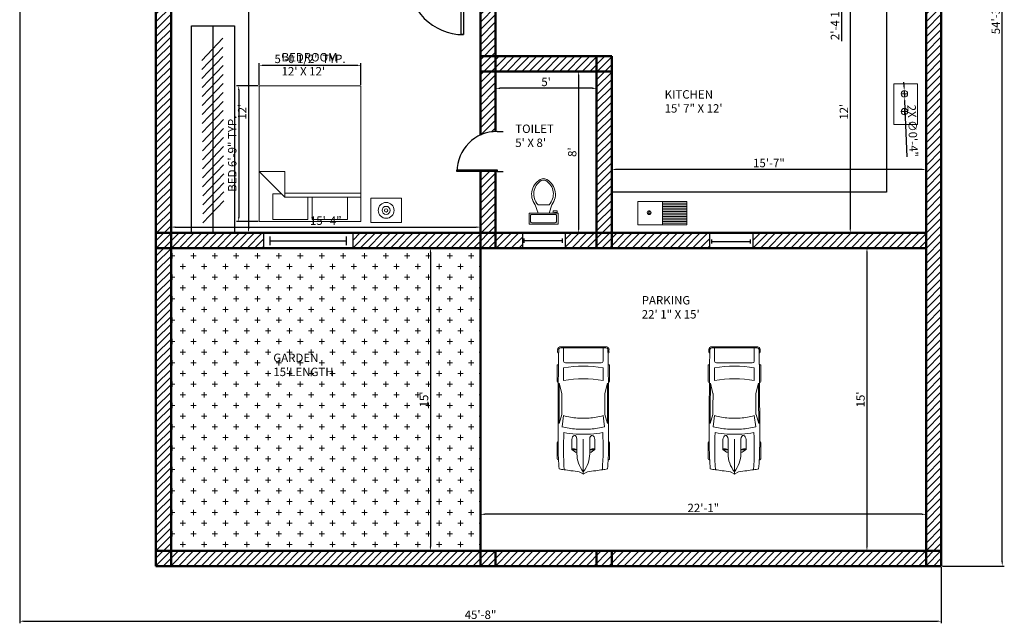
# Model space of a CAD drawing. Units: millimetres. Extents: x 2829 to 4029, y 962 to 1687.
# Tile 5 of 7: x 3444 to 4029, y 962 to 1321. Entities that reach past the tile are written whole.
import ezdxf

# ---------------------------------------------------------------- set-up
doc = ezdxf.new("R2010")
doc.units = ezdxf.units.MM
for name, color, linetype, lineweight in [('A-ANNO-DIMS', 140, 'Continuous', 18), ('A-AREA-IDEN', 190, 'Continuous', 25), ('A-EQPM', 90, 'Continuous', 18), ('A-FLOR-CASE', 90, 'Continuous', 25), ('A-FLOR-CASE-PATT', 90, 'Continuous', 13), ('A-FLOR-FIXT', 90, 'Continuous', 18), ('A-FLOR-FIXT-PATT', 90, 'Continuous', 13), ('A-WALL-PATT', 2, 'Continuous', 13), ('C-PRKG-VEHS', 90, 'Continuous', 18), ('doors', 10, 'Continuous', 25), ('furniture', 90, 'Continuous', 18), ('walls', 50, 'Continuous', 50), ('windows', 30, 'Continuous', 25)]:
    doc.layers.add(name, color=color, linetype=linetype, lineweight=lineweight)
doc.layers.add('L-PLNT-PATT', color=143, linetype='Continuous', lineweight=13, true_color=0x7aafdf)
doc.styles.get("Standard").update_dxf_attribs({"font": 'arial.ttf'})
doc.dimstyles.new('ISO-25', dxfattribs={"dimtxt": 5, "dimasz": 2.5, "dimexe": 1.25, "dimexo": 0.625, "dimtad": 1, "dimdec": 0, "dimlunit": 3, "dimtxsty": 'Standard', "dimcen": 2.5, "dimadec": 0, "dimazin": 0, "dimtfac": 1, "dimtdec": 0, "dimtmove": 0, "dimatfit": 3, "dimfxl": 1, "dimarcsym": 0})

# ---------------------------------------------------------------- blocks, each defined once
blk = doc.blocks.new('*U2')
for p, q in [((0, 0), (0, -6)), ((40, 0), (40, -6))]:
    blk.add_line(p, q)
blk.add_lwpolyline([(0, 0), (0, 40), (1.75, 40), (1.75, 0)], close=True)
blk.add_arc((0, 0), 40, 0, 90)
blk = doc.blocks.new('*U32')
for p, q in [((0, 4), (0, 0)), ((0, 2), (36, 2)), ((36, 4), (36, 0))]:
    blk.add_line(p, q)
blk = doc.blocks.new('*U33')
for p, q in [((0, 4), (0, 0)), ((0, 2), (36, 2)), ((36, 4), (36, 0))]:
    blk.add_line(p, q)
blk = doc.blocks.new('Bed - Queen')
for p, q in [((0, -80.00003), (0, 0)), ((0, 0), (59.99999, 0)), ((59.99999, 0), (59.99999, -80.00003)), ((7.99999, -1.2), (28.79998, -1.2)), ((7.99999, -14.4), (7.99999, -1.2)), ((28.79998, -1.2), (28.79998, -14.4)), ((31.19999, -1.2), (51.99999, -1.2)), ((31.19999, -14.4), (31.19999, -1.2)), ((51.99999, -1.2), (51.99999, -16.4)), ((0, -14.4), (44.8, -14.4)), ((44.8, -16.8), (0, -16.8)), ((59.99999, -29.6), (44.8, -14.4)), ((44.8, -14.4), (44.8, -29.6)), ((51.99999, -16.4), (46.79936, -16.4)), ((44.8, -29.6), (59.99999, -29.6)), ((59.99999, -80.00003), (0, -80.00003))]:
    blk.add_line(p, q)
blk = doc.blocks.new('*U35')
for p, q in [((21.1, 37.4), (21.1, 36.8)), ((46.6, 38.9), (22.4, 38.9)), ((47.8, 37.4), (47.8, 37.4)), ((70, 31.5), (86.4, 29.4)), ((88, 31.9), (74.8, 35.9)), ((134.3, 35.6), (119.3, 31.8)), ((135.5, 37.1), (135.5, 37.4)), ((136.7, 38.9), (160.9, 38.9)), ((138.4, 29.4), (157.2, 29.4)), ((162.1, 37.4), (162.1, 36.8)), ((186.5, 29.4), (167, 29.4)), ((186.5, -33.5), (186.5, 33.5)), ((188.4, -32.8), (188.4, 32.8)), ((32.3, 11.6), (36.1, 17.2)), ((36.1, 17.2), (50.9, 17.2)), ((164.5, 26.4), (164.5, -26.4)), ((3.3, 6.1), (0.1, 0.4)), ((29.8, 9.5), (51.7, 9.5)), ((32.1, 9.5), (32.1, 11.2)), ((58.9, -10.8), (58.9, 10.8)), ((66.6, -10.5), (66.6, 10.5)), ((82.7, 8.5), (82.7, -8.5)), ((186.5, -10.5), (186.5, 10.5)), ((0, 0), (51.7, 0)), ((0.1, -0.4), (3.3, -6.1)), ((29.8, -9.5), (51.7, -9.5)), ((32.1, -9.5), (32.1, -11.2)), ((32.3, -11.6), (36.1, -17.2)), ((36.1, -17.2), (50.9, -17.2)), ((21.1, -37.4), (21.1, -36.8)), ((46.6, -38.9), (22.4, -38.9)), ((47.8, -37.4), (47.8, -37.4)), ((86.4, -29.4), (70, -31.5)), ((88, -31.9), (74.8, -35.9)), ((134.3, -35.6), (119.3, -31.8)), ((135.5, -37.1), (135.5, -37.4)), ((136.7, -38.9), (160.9, -38.9)), ((157.2, -29.4), (138.4, -29.4)), ((162.1, -37.4), (162.1, -36.8)), ((167, -29.4), (186.5, -29.4))]:
    blk.add_line(p, q)
for centre, major_axis, ratio, start_param, end_param in [((266, -27.5), (0, 313.3), 0.842304, 1.367076, 1.39176), ((37.5, -594), (0, -623.3), 0.842304, 3.096046, 3.200911), ((41.2, -490.9), (0, 528.2), 0.842304, 0.00281, 0.075598), ((22.4, 37.4), (0, -1.48), 0.842304, 3.141593, 4.712389), ((64.5, -10555.6), (0, 10593), 0.842304, -0.013397, 0.002797), ((46.6, 37.4), (0, 1.48), 0.842304, -1.570796, 0), ((135.3, 5.4), (0, 81.8), 0.842304, 1.245306, 1.50788), ((64.5, -10555.6), (0, -10591.5), 0.842304, 3.133765, 3.140441), ((149.6, 2.8), (0, -79.6), 0.842304, 4.372215, 4.640744), ((95.8, -3666.4), (0, -3698.2), 0.842304, 3.134049, 3.144098), ((136.7, 37.4), (0, -1.48), 0.842304, 3.141593, 4.712389), ((17.1, 0), (0, 147), 0.842304, 4.511394, 4.913384), ((35.9, 0), (0, 147), 0.842304, 4.511394, 4.913384), ((160.9, 37.4), (0, 1.48), 0.842304, -1.570796, 0), ((167, 26.4), (0, 2.96), 0.842304, 0, 1.570796), ((180.6, 35.8), (0, 2.22), 0.842304, -0.013017, 1.249894), ((64.5, -10556.4), (0, 10595.3), 0.842304, -0.013397, -0.013017), ((184, 32.8), (0, -5.25), 0.842304, 1.570796, 3.128196), ((184, 33.5), (0, -2.96), 0.842304, 1.570796, 3.128196), ((-204.5, 52.4), (0, -251), 0.842304, 1.385369, 1.434372), ((259.2, -27.5), (0, -305.3), 0.842304, 4.528606, 4.561838), ((13, 17), (0, 27.4), 0.842304, 4.435146, 4.718221), ((14.2, 17), (0, 27.4), 0.842304, 4.435146, 4.718221), ((50.8, 13.3), (6.34, -0.36), 0.603834, -1.395552, 1.581315), ((134.4, 5.4), (0, -89.8), 0.842304, 4.449482, 4.652344), ((0.6, 0), (0, -0.74), 0.842304, 4.131459, 5.293319), ((29.8, -46.7), (0, 56.2), 0.842304, 0, 0.590319), ((32.7, 11.2), (0, 0.74), 0.842304, 0.879714, 1.570796), ((-204.5, -52.4), (0, 251), 0.842304, -1.434372, -1.385369), ((29.8, 46.7), (0, 56.2), 0.842304, 2.551274, 3.141593), ((32.7, -11.2), (0, -0.74), 0.842304, 4.712389, 5.403472), ((13, -17), (0, -27.4), 0.842304, 1.564964, 1.848039), ((14.2, -17), (0, -27.4), 0.842304, 1.564964, 1.848039), ((134.4, -5.4), (0, -89.8), 0.842304, -1.510751, -1.307889), ((135.3, -5.4), (0, -81.8), 0.842304, -1.50788, -1.245306), ((149.6, -2.8), (0, -79.6), 0.842304, -1.499151, -1.230623), ((259.2, 27.5), (0, 305.3), 0.842304, 1.721348, 1.754579), ((266, 27.5), (0, 313.3), 0.842304, 1.749832, 1.774517), ((37.5, 594), (0, -623.3), 0.842304, -0.059319, 0.045547), ((167, -26.4), (0, -2.96), 0.842304, 4.712389, 6.283185), ((41.2, 490.9), (0, -528.2), 0.842304, -0.075598, -0.00281), ((22.4, -37.4), (0, 1.48), 0.842304, 1.570796, 3.141593), ((64.5, 10555.6), (0, 10593), 0.842304, 3.138796, 3.15499), ((46.6, -37.4), (0, -1.48), 0.842304, 0, 1.570796), ((64.5, 10555.6), (0, -10591.5), 0.842304, 0.001152, 0.007828), ((95.8, 3666.4), (0, -3698.2), 0.842304, -0.002505, 0.007544), ((136.7, -37.4), (0, -1.48), 0.842304, -1.570796, 0), ((160.9, -37.4), (0, 1.48), 0.842304, 3.141593, 4.712389), ((180.6, -35.8), (0, -2.22), 0.842304, -1.249894, 0.013017), ((64.5, 10556.4), (0, 10595.3), 0.842304, 3.15461, 3.15499), ((184, -32.8), (0, -5.25), 0.842304, 0.013397, 1.570796), ((184, -33.5), (0, 2.96), 0.842304, 3.15499, 4.712389)]:
    blk.add_ellipse(centre, major_axis=major_axis, ratio=ratio, start_param=start_param, end_param=end_param)
at = {"extrusion": (0, 0, -1)}
blk.add_ellipse((50.8, -13.3), major_axis=(6.34, 0.36), ratio=0.603834, start_param=-1.395552, end_param=1.581315, dxfattribs=at)
blk = doc.blocks.new('Toilet - top')
for p, q in [((9.5, -6), (9.5, -2)), ((-10, -8.5), (-8, -8.5)), ((-10, -9.5), (-10, -8.5)), ((-7, -9.5), (-10, -9.5)), ((-8, -8.5), (-8, -8)), ((-7, -8), (-7, -9.5)), ((-4, -8), (-6, -14)), ((4, -14), (-4, -14)), ((4, -8), (6, -14))]:
    blk.add_line(p, q)
blk.add_lwpolyline([(10.5, -8), (10.5, 0), (-10.5, 0), (-10.5, -8)], close=True)
for points in [[(-9.5, -2), (-9.5, -6)], [(8.5, -1), (-8.5, -1)], [(-8.5, -7), (8.5, -7)]]:
    blk.add_lwpolyline(points)
for centre, radius, start, end in [((-8.62, -1.88), 0.884, 81.8699, 188.1301), ((-8.62, -6.12), 0.884, 171.8699, 278.1301), ((8.62, -1.88), 0.884, 351.8699, 98.1301), ((8.62, -6.12), 0.884, 261.8699, 8.1301), ((3.52, -21.58), 12.17, 141.46911, 247.97143), ((4.2, -21.82), 11.33, 136.36773, 238.94682), ((-3.52, -21.58), 12.17, 292.02843, 38.53071), ((-4.2, -21.82), 11.33, 301.05301, 43.63209), ((0, -27.88), 4, 245.73182, 294.26817), ((0, -29), 4, 254.86053, 285.13947)]:
    blk.add_arc(centre, radius, start, end)
blk = doc.blocks.new('*D42')
at = {"layer": 'A-ANNO-DIMS', "color": 0, "lineweight": -2, "transparency": 16777216}
for p, q in [((3776.63, 1290.27), (3777.26, 1290.27)), ((3776.01, 1287.77), (3776.01, 1196.77)), ((3776.63, 1194.27), (3777.26, 1194.27))]:
    blk.add_line(p, q, dxfattribs=at)
at = {"layer": 'A-ANNO-DIMS', "color": 0, "transparency": 16777216}
for points in [[(3775.59, 1287.77), (3776.42, 1287.77), (3776.01, 1290.27)], [(3775.59, 1196.77), (3776.42, 1196.77), (3776.01, 1194.27)]]:
    blk.add_solid(points, dxfattribs=at)
at = {"layer": 'Defpoints', "color": 0, "transparency": 16777216}
for p in [(3776.01, 1290.27), (3776.01, 1194.27), (3776.01, 1194.27)]:
    blk.add_point(p, dxfattribs=at)
at = {"layer": 'A-ANNO-DIMS', "color": 0, "transparency": 16777216, "insert": (3772.83, 1242.27), "char_height": 5, "attachment_point": 5, "rotation": 90}
blk.add_mtext("8'", dxfattribs=at)
blk = doc.blocks.new('*D43')
at = {"layer": 'A-ANNO-DIMS', "color": 0, "lineweight": -2, "transparency": 16777216}
for p, q in [((3726.66, 1282.83), (3726.66, 1278.94)), ((3786.66, 1282.83), (3786.66, 1278.94)), ((3784.16, 1280.19), (3729.16, 1280.19))]:
    blk.add_line(p, q, dxfattribs=at)
at = {"layer": 'A-ANNO-DIMS', "color": 0, "transparency": 16777216}
for points in [[(3729.16, 1280.61), (3729.16, 1279.78), (3726.66, 1280.19)], [(3784.16, 1280.61), (3784.16, 1279.78), (3786.66, 1280.19)]]:
    blk.add_solid(points, dxfattribs=at)
at = {"layer": 'Defpoints', "color": 0, "transparency": 16777216}
for p in [(3726.66, 1283.46), (3786.66, 1283.46), (3726.66, 1280.19)]:
    blk.add_point(p, dxfattribs=at)
at = {"layer": 'A-ANNO-DIMS', "color": 0, "transparency": 16777216, "insert": (3756.66, 1283.36), "char_height": 5, "attachment_point": 5}
blk.add_mtext("5'", dxfattribs=at)
blk = doc.blocks.new('*D44')
at = {"layer": 'A-ANNO-DIMS', "color": 0, "lineweight": -2, "transparency": 16777216}
for p, q in [((3947.43, 1182.77), (3947.43, 1007.77)), ((3947.78, 1185.27), (3948.68, 1185.27)), ((3947.78, 1005.27), (3948.68, 1005.27))]:
    blk.add_line(p, q, dxfattribs=at)
at = {"layer": 'A-ANNO-DIMS', "color": 0, "transparency": 16777216}
for points in [[(3947.01, 1182.77), (3947.84, 1182.77), (3947.43, 1185.27)], [(3947.01, 1007.77), (3947.84, 1007.77), (3947.43, 1005.27)]]:
    blk.add_solid(points, dxfattribs=at)
at = {"layer": 'Defpoints', "color": 0, "transparency": 16777216}
for p in [(3947.15, 1185.27), (3947.15, 1005.27), (3947.43, 1005.27)]:
    blk.add_point(p, dxfattribs=at)
at = {"layer": 'A-ANNO-DIMS', "color": 0, "transparency": 16777216, "insert": (3944.25, 1095.27), "char_height": 5, "attachment_point": 5, "rotation": 90}
blk.add_mtext("15'", dxfattribs=at)
blk = doc.blocks.new('*D45')
at = {"layer": 'A-ANNO-DIMS', "color": 0, "lineweight": -2, "transparency": 16777216}
for p, q in [((3717.66, 1027.63), (3717.66, 1028.25)), ((3980.16, 1027), (3720.16, 1027)), ((3982.66, 1027.63), (3982.66, 1028.25))]:
    blk.add_line(p, q, dxfattribs=at)
at = {"layer": 'A-ANNO-DIMS', "color": 0, "transparency": 16777216}
for points in [[(3720.16, 1027.42), (3720.16, 1026.59), (3717.66, 1027)], [(3980.16, 1027.42), (3980.16, 1026.59), (3982.66, 1027)]]:
    blk.add_solid(points, dxfattribs=at)
at = {"layer": 'Defpoints', "color": 0, "transparency": 16777216}
for p in [(3717.66, 1027), (3717.66, 1027), (3982.66, 1027)]:
    blk.add_point(p, dxfattribs=at)
at = {"layer": 'A-ANNO-DIMS', "color": 0, "transparency": 16777216, "insert": (3850.16, 1030.14), "char_height": 5, "attachment_point": 5}
blk.add_mtext('22\'-1"', dxfattribs=at)
blk = doc.blocks.new('*D46')
at = {"layer": 'A-ANNO-DIMS', "color": 0, "lineweight": -2, "transparency": 16777216}
for p, q in [((3685.57, 1185.27), (3689.13, 1185.27)), ((3687.88, 1182.77), (3687.88, 1007.77)), ((3685.57, 1005.27), (3689.13, 1005.27))]:
    blk.add_line(p, q, dxfattribs=at)
at = {"layer": 'A-ANNO-DIMS', "color": 0, "transparency": 16777216}
for points in [[(3687.47, 1182.77), (3688.3, 1182.77), (3687.88, 1185.27)], [(3687.47, 1007.77), (3688.3, 1007.77), (3687.88, 1005.27)]]:
    blk.add_solid(points, dxfattribs=at)
at = {"layer": 'Defpoints', "color": 0, "transparency": 16777216}
for p in [(3684.95, 1185.27), (3684.95, 1005.27), (3687.88, 1005.27)]:
    blk.add_point(p, dxfattribs=at)
at = {"layer": 'A-ANNO-DIMS', "color": 0, "transparency": 16777216, "insert": (3684.71, 1095.27), "char_height": 5, "attachment_point": 5, "rotation": 90}
blk.add_mtext("15'", dxfattribs=at)
blk = doc.blocks.new('*D47')
at = {"layer": 'A-ANNO-DIMS', "color": 0, "lineweight": -2, "transparency": 16777216}
for p, q in [((3579.16, 1338.27), (3580.98, 1338.27)), ((3579.73, 1335.77), (3579.73, 1196.77)), ((3579.16, 1194.27), (3580.98, 1194.27))]:
    blk.add_line(p, q, dxfattribs=at)
at = {"layer": 'A-ANNO-DIMS', "color": 0, "transparency": 16777216}
for points in [[(3579.31, 1335.77), (3580.15, 1335.77), (3579.73, 1338.27)], [(3579.31, 1196.77), (3580.15, 1196.77), (3579.73, 1194.27)]]:
    blk.add_solid(points, dxfattribs=at)
at = {"layer": 'Defpoints', "color": 0, "transparency": 16777216}
for p in [(3578.53, 1338.27), (3578.53, 1194.27), (3579.73, 1194.27)]:
    blk.add_point(p, dxfattribs=at)
at = {"layer": 'A-ANNO-DIMS', "color": 0, "transparency": 16777216, "insert": (3576.59, 1266.27), "char_height": 5, "attachment_point": 5, "rotation": 90}
blk.add_mtext("12'", dxfattribs=at)
blk = doc.blocks.new('*D48')
at = {"layer": 'A-ANNO-DIMS', "color": 0, "lineweight": -2, "transparency": 16777216}
for p, q in [((3533.66, 1199.99), (3533.66, 1196.45)), ((3536.16, 1197.7), (3715.16, 1197.7)), ((3717.66, 1198.33), (3717.66, 1198.95))]:
    blk.add_line(p, q, dxfattribs=at)
at = {"layer": 'A-ANNO-DIMS', "color": 0, "transparency": 16777216}
for points in [[(3536.16, 1198.12), (3536.16, 1197.28), (3533.66, 1197.7)], [(3715.16, 1198.12), (3715.16, 1197.28), (3717.66, 1197.7)]]:
    blk.add_solid(points, dxfattribs=at)
at = {"layer": 'Defpoints', "color": 0, "transparency": 16777216}
for p in [(3533.66, 1200.61), (3717.66, 1197.7), (3717.66, 1197.7)]:
    blk.add_point(p, dxfattribs=at)
at = {"layer": 'A-ANNO-DIMS', "color": 0, "transparency": 16777216, "insert": (3625.66, 1200.88), "char_height": 5, "attachment_point": 5}
blk.add_mtext('15\'-4"', dxfattribs=at)
blk = doc.blocks.new('*D55')
at = {"layer": 'A-ANNO-DIMS', "color": 0, "lineweight": -2, "transparency": 16777216}
for p, q in [((3937.54, 1338.27), (3936.26, 1338.27)), ((3937.51, 1335.77), (3937.51, 1196.77)), ((3937.54, 1194.27), (3936.26, 1194.27))]:
    blk.add_line(p, q, dxfattribs=at)
at = {"layer": 'A-ANNO-DIMS', "color": 0, "transparency": 16777216}
for points in [[(3937.1, 1335.77), (3937.93, 1335.77), (3937.51, 1338.27)], [(3937.1, 1196.77), (3937.93, 1196.77), (3937.51, 1194.27)]]:
    blk.add_solid(points, dxfattribs=at)
at = {"layer": 'Defpoints', "color": 0, "transparency": 16777216}
for p in [(3938.16, 1338.27), (3937.51, 1194.27), (3938.16, 1194.27)]:
    blk.add_point(p, dxfattribs=at)
at = {"layer": 'A-ANNO-DIMS', "color": 0, "transparency": 16777216, "insert": (3934.38, 1266.27), "char_height": 5, "attachment_point": 5, "rotation": 90}
blk.add_mtext("12'", dxfattribs=at)
blk = doc.blocks.new('*D56')
at = {"layer": 'A-ANNO-DIMS', "color": 0, "lineweight": -2, "transparency": 16777216}
for p, q in [((3795.66, 1231.66), (3795.66, 1230.72)), ((3980.16, 1231.97), (3798.16, 1231.97)), ((3982.66, 1231.66), (3982.66, 1230.72))]:
    blk.add_line(p, q, dxfattribs=at)
at = {"layer": 'A-ANNO-DIMS', "color": 0, "transparency": 16777216}
for points in [[(3798.16, 1232.39), (3798.16, 1231.55), (3795.66, 1231.97)], [(3980.16, 1232.39), (3980.16, 1231.55), (3982.66, 1231.97)]]:
    blk.add_solid(points, dxfattribs=at)
at = {"layer": 'Defpoints', "color": 0, "transparency": 16777216}
for p in [(3795.66, 1232.29), (3795.66, 1231.97), (3982.66, 1232.29)]:
    blk.add_point(p, dxfattribs=at)
at = {"layer": 'A-ANNO-DIMS', "color": 0, "transparency": 16777216, "insert": (3889.16, 1235.15), "char_height": 5, "attachment_point": 5}
blk.add_mtext('15\'-7"', dxfattribs=at)
blk = doc.blocks.new('COOKTOP-BURNER-LARGE')
for p, q in [((0, 1.91), (3.83, 1.91)), ((1.91, 3.83), (1.91, 0))]:
    blk.add_line(p, q)
blk.add_circle((1.91, 1.91), 1.91)
blk = doc.blocks.new('*D68')
at = {"layer": 'A-ANNO-DIMS', "color": 0, "lineweight": -2, "transparency": 16777216}
for p, q in [((3923.13, 1382.67), (3933.53, 1382.67)), ((3932.28, 1380.17), (3932.28, 1356.73)), ((3923.13, 1354.23), (3933.53, 1354.23)), ((3932.28, 1354.23), (3932.28, 1308.27))]:
    blk.add_line(p, q, dxfattribs=at)
at = {"layer": 'A-ANNO-DIMS', "color": 0, "transparency": 16777216}
for points in [[(3931.86, 1380.17), (3932.7, 1380.17), (3932.28, 1382.67)], [(3931.86, 1356.73), (3932.7, 1356.73), (3932.28, 1354.23)]]:
    blk.add_solid(points, dxfattribs=at)
at = {"layer": 'Defpoints', "color": 0, "transparency": 16777216}
for p in [(3922.51, 1382.67), (3922.51, 1354.23), (3932.28, 1354.23)]:
    blk.add_point(p, dxfattribs=at)
at = {"layer": 'A-ANNO-DIMS', "color": 0, "transparency": 16777216, "insert": (3929.07, 1330), "char_height": 5, "attachment_point": 5, "rotation": 90}
blk.add_mtext('2\'-4 1/2" TYP.', dxfattribs=at)
blk = doc.blocks.new('*D71')
at = {"layer": 'A-ANNO-DIMS', "color": 0, "lineweight": -2, "transparency": 16777216}
for p, q in [((3585.37, 1281.74), (3572.63, 1281.74)), ((3573.88, 1279.24), (3573.88, 1203.47)), ((3585.37, 1200.97), (3572.63, 1200.97))]:
    blk.add_line(p, q, dxfattribs=at)
at = {"layer": 'A-ANNO-DIMS', "color": 0, "transparency": 16777216}
for points in [[(3573.47, 1279.24), (3574.3, 1279.24), (3573.88, 1281.74)], [(3573.47, 1203.47), (3574.3, 1203.47), (3573.88, 1200.97)]]:
    blk.add_solid(points, dxfattribs=at)
at = {"layer": 'Defpoints', "color": 0, "transparency": 16777216}
for p in [(3586, 1281.74), (3573.88, 1200.97), (3586, 1200.97)]:
    blk.add_point(p, dxfattribs=at)
at = {"layer": 'A-ANNO-DIMS', "color": 0, "transparency": 16777216, "insert": (3570.7, 1241.35), "char_height": 5, "attachment_point": 5, "rotation": 90}
blk.add_mtext('BED 6\'-9" TYP.', dxfattribs=at)
blk = doc.blocks.new('*D72')
at = {"layer": 'A-ANNO-DIMS', "color": 0, "lineweight": -2, "transparency": 16777216}
for p, q in [((3586, 1282.36), (3586, 1295.1)), ((3644.08, 1293.85), (3588.5, 1293.85)), ((3646.58, 1282.36), (3646.58, 1295.1))]:
    blk.add_line(p, q, dxfattribs=at)
at = {"layer": 'A-ANNO-DIMS', "color": 0, "transparency": 16777216}
for points in [[(3588.5, 1294.27), (3588.5, 1293.44), (3586, 1293.85)], [(3644.08, 1294.27), (3644.08, 1293.44), (3646.58, 1293.85)]]:
    blk.add_solid(points, dxfattribs=at)
at = {"layer": 'Defpoints', "color": 0, "transparency": 16777216}
for p in [(3586, 1293.85), (3586, 1281.74), (3646.58, 1281.74)]:
    blk.add_point(p, dxfattribs=at)
at = {"layer": 'A-ANNO-DIMS', "color": 0, "transparency": 16777216, "insert": (3616.29, 1297.06), "char_height": 5, "attachment_point": 5}
blk.add_mtext('5\'-0 1/2" TYP.', dxfattribs=at)
blk = doc.blocks.new('*D92')
at = {"layer": 'A-ANNO-DIMS', "color": 0, "lineweight": -2, "transparency": 16777216}
for p, q in [((3443.66, 1337.65), (3443.66, 962.22)), ((3991.66, 995.65), (3991.66, 962.22)), ((3446.16, 963.47), (3989.16, 963.47))]:
    blk.add_line(p, q, dxfattribs=at)
at = {"layer": 'A-ANNO-DIMS', "color": 0, "transparency": 16777216}
for points in [[(3446.16, 963.89), (3446.16, 963.05), (3443.66, 963.47)], [(3989.16, 963.89), (3989.16, 963.05), (3991.66, 963.47)]]:
    blk.add_solid(points, dxfattribs=at)
at = {"layer": 'Defpoints', "color": 0, "transparency": 16777216}
for p in [(3443.66, 1338.27), (3991.66, 996.27), (3991.66, 963.47)]:
    blk.add_point(p, dxfattribs=at)
at = {"layer": 'A-ANNO-DIMS', "color": 0, "transparency": 16777216, "insert": (3717.66, 966.65), "char_height": 5, "attachment_point": 5}
blk.add_mtext('45\'-8"', dxfattribs=at)
blk = doc.blocks.new('*D93')
at = {"layer": 'A-ANNO-DIMS', "color": 0, "lineweight": -2, "transparency": 16777216}
for p, q in [((3992.28, 1647.27), (4029.11, 1647.27)), ((4027.86, 998.77), (4027.86, 1644.77)), ((3992.28, 996.27), (4029.11, 996.27))]:
    blk.add_line(p, q, dxfattribs=at)
at = {"layer": 'A-ANNO-DIMS', "color": 0, "transparency": 16777216}
for points in [[(4027.44, 1644.77), (4028.28, 1644.77), (4027.86, 1647.27)], [(4027.44, 998.77), (4028.28, 998.77), (4027.86, 996.27)]]:
    blk.add_solid(points, dxfattribs=at)
at = {"layer": 'Defpoints', "color": 0, "transparency": 16777216}
for p in [(3991.66, 1647.27), (4027.86, 1647.27), (3991.66, 996.27)]:
    blk.add_point(p, dxfattribs=at)
at = {"layer": 'A-ANNO-DIMS', "color": 0, "transparency": 16777216, "insert": (4024.68, 1321.77), "char_height": 5, "attachment_point": 5, "rotation": 90}
blk.add_mtext('54\'-3"', dxfattribs=at)
blk = doc.blocks.new('*D97')
at = {"layer": 'A-ANNO-DIMS', "color": 0, "lineweight": -2, "transparency": 16777216}
for p, q in [((3969.52, 1281.3), (3969.41, 1283.8)), ((3969.63, 1278.8), (3969.8, 1274.97)), ((3971.37, 1239.47), (3969.91, 1272.48))]:
    blk.add_line(p, q, dxfattribs=at)
at = {"layer": 'A-ANNO-DIMS', "color": 0, "transparency": 16777216}
for points in [[(3969.94, 1281.32), (3969.1, 1281.28), (3969.63, 1278.8)], [(3970.33, 1272.5), (3969.49, 1272.46), (3969.8, 1274.97)]]:
    blk.add_solid(points, dxfattribs=at)
at = {"layer": 'Defpoints', "color": 0, "transparency": 16777216}
for p in [(3969.63, 1278.8), (3969.8, 1274.97)]:
    blk.add_point(p, dxfattribs=at)
at = {"layer": 'A-ANNO-DIMS', "color": 0, "transparency": 16777216, "insert": (3974.01, 1254.87), "char_height": 5, "attachment_point": 5, "rotation": 272.53976}
blk.add_mtext('2X ∅0\'-4"', dxfattribs=at)

msp = doc.modelspace()

# ---------------------------------------------------------------- hatches: boundary and pattern name
at = {"layer": 'A-FLOR-CASE-PATT'}
h = msp.add_hatch(dxfattribs=at)
h.set_pattern_fill('ANSI31', color=256, scale=1.17252, angle=1.417, style=0)
h.paths.add_polyline_path([(3551.96, 1297.28), (3552.59, 1195.34), (3565.09, 1208.47), (3564.47, 1310.42)])
at = {"layer": 'A-FLOR-FIXT-PATT'}
h = msp.add_hatch(dxfattribs=at)
h.set_pattern_fill('ANSI31', color=256, scale=0.314961, angle=-45, style=0)
h.paths.add_polyline_path([(3840.43, 1212.95), (3825.8, 1212.95), (3825.8, 1198.95), (3840.43, 1198.95)])
at = {"layer": 'A-WALL-PATT'}
h = msp.add_hatch(dxfattribs=at)
h.set_pattern_fill('ANSI31', color=256)
h.set_pattern_definition([(45, (-1090.0668, 570.9627), (-2.245064, 2.245064), [])])
h.paths.add_polyline_path([(3524.66, 1494.27), (3452.66, 1494.27), (3452.66, 1485.27), (3524.66, 1485.27)])
h.paths.add_polyline_path([(3452.66, 1494.27), (3443.66, 1494.27), (3443.66, 1485.27), (3452.66, 1485.27)])
h.paths.add_polyline_path([(3452.66, 1485.27), (3443.66, 1485.27), (3443.66, 1347.27), (3452.66, 1347.27)])
h.paths.add_polyline_path([(3533.66, 1433.28), (3524.66, 1433.28), (3524.66, 1400.41), (3533.66, 1400.41)])
h.paths.add_polyline_path([(3524.66, 1347.27), (3452.66, 1347.27), (3452.66, 1338.27), (3524.66, 1338.27)])
h.paths.add_polyline_path([(3452.66, 1347.27), (3443.66, 1347.27), (3443.66, 1338.27), (3452.66, 1338.27)])
h.paths.add_polyline_path([(3533.66, 1347.27), (3524.66, 1347.27), (3524.66, 1338.27), (3533.66, 1338.27)])
h.paths.add_polyline_path([(3674.61, 1345.02), (3674.61, 1347.27), (3533.66, 1347.27), (3533.66, 1338.27), (3675.31, 1338.27, -0.051672)])
h.paths.add_polyline_path([(3533.66, 1638.27), (3524.66, 1638.27), (3524.66, 1494.27), (3533.66, 1494.27)])
h.paths.add_polyline_path([(3533.66, 1494.27), (3524.66, 1494.27), (3524.66, 1485.27), (3533.66, 1485.27)])
h.paths.add_polyline_path([(3643.72, 1494.27), (3533.66, 1494.27), (3533.66, 1485.27), (3643.72, 1485.27), (3643.72, 1487.41)])
h.paths.add_polyline_path([(3533.66, 1647.27), (3524.66, 1647.27), (3524.66, 1638.27), (3533.66, 1638.27)])
h.paths.add_polyline_path([(3573.07, 1647.27), (3533.66, 1647.27), (3533.66, 1638.27), (3573.07, 1638.27)])
h.paths.add_polyline_path([(3684.66, 1647.27), (3622.32, 1647.27), (3622.32, 1638.27), (3684.66, 1638.27)])
h.paths.add_polyline_path([(3693.66, 1647.27), (3684.66, 1647.27), (3684.66, 1638.27), (3693.66, 1638.27)])
h.paths.add_polyline_path([(3693.66, 1638.27), (3684.66, 1638.27), (3684.66, 1601.42, -0.100401), (3693.66, 1604.42)])
h.paths.add_polyline_path([(3693.66, 1580.73), (3684.66, 1580.73), (3684.66, 1542.27), (3693.66, 1542.27)])
h.paths.add_polyline_path([(3693.66, 1542.27), (3684.66, 1542.27), (3684.66, 1533.27), (3693.66, 1533.27)])
h.paths.add_polyline_path([(3693.66, 1533.27), (3684.66, 1533.27), (3684.66, 1494.27), (3693.66, 1494.27)])
h.paths.add_polyline_path([(3693.66, 1494.27), (3684.66, 1494.27), (3684.66, 1485.27), (3693.66, 1485.27)])
h.paths.add_polyline_path([(3684.66, 1494.27), (3675.91, 1494.27, -0.052559), (3676.64, 1487.41), (3676.64, 1485.27), (3684.66, 1485.27)])
h.paths.add_polyline_path([(3753.66, 1542.27), (3693.66, 1542.27), (3693.66, 1533.27), (3753.66, 1533.27)])
h.paths.add_polyline_path([(3762.66, 1542.27), (3753.66, 1542.27), (3753.66, 1533.27), (3762.66, 1533.27)])
h.paths.add_polyline_path([(3762.66, 1638.27), (3753.66, 1638.27), (3753.66, 1542.27), (3762.66, 1542.27)])
h.paths.add_polyline_path([(3762.66, 1647.27), (3753.66, 1647.27), (3753.66, 1638.27), (3762.66, 1638.27)])
h.paths.add_polyline_path([(3753.66, 1647.27), (3733.82, 1647.27), (3733.82, 1638.27), (3753.66, 1638.27)])
h.paths.add_polyline_path([(3706.41, 1647.27), (3693.66, 1647.27), (3693.66, 1638.27), (3706.41, 1638.27)])
h.paths.add_polyline_path([(3822.66, 1647.27), (3804.07, 1647.27), (3804.07, 1638.27), (3822.66, 1638.27)])
h.paths.add_polyline_path([(3778.61, 1647.27), (3762.66, 1647.27), (3762.66, 1638.27), (3778.61, 1638.27)])
h.paths.add_polyline_path([(3822.66, 1542.27), (3762.66, 1542.27), (3762.66, 1533.27), (3822.66, 1533.27)])
h.paths.add_polyline_path([(3831.66, 1542.27), (3822.66, 1542.27), (3822.66, 1533.27), (3831.66, 1533.27)])
h.paths.add_polyline_path([(3831.66, 1587.4), (3822.66, 1587.4), (3822.66, 1542.27), (3831.66, 1542.27)])
h.paths.add_polyline_path([(3831.66, 1638.27), (3822.66, 1638.27), (3822.66, 1611.22, -0.098322), (3831.66, 1608.9)])
h.paths.add_polyline_path([(3831.66, 1647.27), (3822.66, 1647.27), (3822.66, 1638.27), (3831.66, 1638.27)])
h.paths.add_polyline_path([(3883.77, 1647.27), (3831.66, 1647.27), (3831.66, 1638.27), (3883.77, 1638.27)])
h.paths.add_polyline_path([(3982.66, 1647.27), (3934.96, 1647.27), (3934.96, 1638.27), (3982.66, 1638.27)])
h.paths.add_polyline_path([(3991.66, 1647.27), (3982.66, 1647.27), (3982.66, 1638.27), (3991.66, 1638.27)])
h.paths.add_polyline_path([(3991.66, 1638.27), (3982.66, 1638.27), (3982.66, 1494.27), (3991.66, 1494.27)])
h.paths.add_polyline_path([(3991.66, 1494.27), (3982.66, 1494.27), (3982.66, 1485.27), (3991.66, 1485.27)])
h.paths.add_polyline_path([(3982.66, 1494.27), (3831.66, 1494.27), (3831.66, 1485.27), (3982.66, 1485.27)])
h.paths.add_polyline_path([(3831.66, 1494.27), (3822.66, 1494.27), (3822.66, 1485.27), (3831.66, 1485.27)])
h.paths.add_polyline_path([(3991.66, 1485.27), (3982.66, 1485.27), (3982.66, 1463.05, -0.057246), (3990.12, 1463.9), (3991.66, 1463.9)])
h.paths.add_polyline_path([(3991.66, 1430.98), (3990.12, 1430.98), (3982.66, 1430.98), (3982.66, 1347.27), (3991.66, 1347.27)])
h.paths.add_polyline_path([(3982.66, 1347.27), (3786.66, 1347.27), (3786.66, 1338.27), (3982.66, 1338.27)])
h.paths.add_polyline_path([(3991.66, 1347.27), (3982.66, 1347.27), (3982.66, 1338.27), (3991.66, 1338.27)])
h.paths.add_polyline_path([(3991.66, 1338.27), (3982.66, 1338.27), (3982.66, 1005.27), (3991.66, 1005.27)])
h.paths.add_polyline_path([(3982.66, 1194.27), (3879.62, 1194.27), (3879.62, 1185.27), (3982.66, 1185.27)])
h.paths.add_polyline_path([(3853.79, 1194.27), (3795.66, 1194.27), (3795.66, 1185.27), (3853.79, 1185.27)])
h.paths.add_polyline_path([(3795.66, 1194.27), (3786.66, 1194.27), (3786.66, 1185.27), (3795.66, 1185.27)])
h.paths.add_polyline_path([(3795.66, 1290.27), (3786.66, 1290.27), (3786.66, 1194.27), (3795.66, 1194.27)])
h.paths.add_polyline_path([(3726.66, 1230.69), (3717.66, 1230.69), (3717.66, 1194.27), (3726.66, 1194.27)])
h.paths.add_polyline_path([(3726.66, 1194.27), (3717.66, 1194.27), (3717.66, 1185.27), (3726.66, 1185.27)])
h.paths.add_polyline_path([(3742.53, 1194.27), (3726.66, 1194.27), (3726.66, 1185.27), (3742.53, 1185.27)])
h.paths.add_polyline_path([(3786.66, 1194.27), (3767.92, 1194.27), (3767.92, 1185.27), (3786.66, 1185.27)])
h.paths.add_polyline_path([(3726.66, 1290.27), (3717.66, 1290.27), (3717.66, 1252.42, -0.097806), (3726.66, 1254.54)])
h.paths.add_polyline_path([(3726.66, 1299.27), (3717.66, 1299.27), (3717.66, 1290.27), (3726.66, 1290.27)])
h.paths.add_polyline_path([(3786.66, 1299.27), (3726.66, 1299.27), (3726.66, 1290.27), (3786.66, 1290.27)])
h.paths.add_polyline_path([(3795.66, 1299.27), (3786.66, 1299.27), (3786.66, 1290.27), (3795.66, 1290.27)])
h.paths.add_polyline_path([(3726.66, 1338.27), (3717.66, 1338.27), (3717.66, 1299.27), (3726.66, 1299.27)])
h.paths.add_polyline_path([(3717.66, 1194.27), (3641.7, 1194.27), (3641.7, 1185.27), (3717.66, 1185.27)])
h.paths.add_polyline_path([(3588.68, 1194.27), (3533.66, 1194.27), (3533.66, 1185.27), (3588.68, 1185.27)])
h.paths.add_polyline_path([(3533.66, 1194.27), (3524.66, 1194.27), (3524.66, 1185.27), (3533.66, 1185.27)])
h.paths.add_polyline_path([(3533.66, 1338.27), (3524.66, 1338.27), (3524.66, 1194.27), (3533.66, 1194.27)])
h.paths.add_polyline_path([(3533.66, 1185.27), (3524.66, 1185.27), (3524.66, 1005.27), (3533.66, 1005.27)])
h.paths.add_polyline_path([(3717.66, 1005.27), (3533.66, 1005.27), (3533.66, 996.27), (3717.66, 996.27)])
h.paths.add_polyline_path([(3726.66, 1005.27), (3717.66, 1005.27), (3717.66, 996.27), (3726.66, 996.27)])
h.paths.add_polyline_path([(3533.66, 1005.27), (3524.66, 1005.27), (3524.66, 996.27), (3533.66, 996.27)])
h.paths.add_polyline_path([(3786.66, 1005.27), (3726.66, 1005.27), (3726.66, 996.27), (3786.66, 996.27)])
h.paths.add_polyline_path([(3982.66, 1005.27), (3795.66, 1005.27), (3795.66, 996.27), (3982.66, 996.27)])
h.paths.add_polyline_path([(3795.66, 1005.27), (3786.66, 1005.27), (3786.66, 996.27), (3795.66, 996.27)])
h.paths.add_polyline_path([(3991.66, 1005.27), (3982.66, 1005.27), (3982.66, 996.27), (3991.66, 996.27)])
at = {"layer": 'L-PLNT-PATT'}
h = msp.add_hatch(dxfattribs=at)
h.set_pattern_fill('CROSS', color=256)
h.set_pattern_definition([(0, (-1090.067, 570.963), (6.35, 6.35), [3.175, -9.525]), (90, (-1088.4793, 569.375), (-6.35, 6.35), [3.175, -9.525])])
h.paths.add_polyline_path([(3717.66, 1185.27), (3533.66, 1185.27), (3533.66, 1005.27), (3717.66, 1005.27)])

# ---------------------------------------------------------------- linework, layer by layer
at = {"layer": 'A-EQPM'}
msp.add_lwpolyline([(3963.34, 1282.79), (3977.54, 1282.79), (3977.54, 1258.72), (3963.34, 1258.72)], close=True, dxfattribs=at)
at = {"layer": 'A-FLOR-CASE'}
for p, q in [((3959.05, 1338.27), (3959.05, 1218.45)), ((3558.59, 1317.32), (3558.59, 1194.27)), ((3959.05, 1218.45), (3795.66, 1218.45))]:
    msp.add_line(p, q, dxfattribs=at)
msp.add_lwpolyline([(3545.73, 1317.32), (3571.44, 1317.32), (3571.44, 1194.27), (3545.73, 1194.27)], close=True, dxfattribs=at)
at = {"layer": 'A-FLOR-FIXT'}
msp.add_line((3825.8, 1212.95), (3825.8, 1199.14), dxfattribs=at)
msp.add_lwpolyline([(3811.16, 1212.95), (3840.43, 1212.95), (3840.43, 1199.14), (3811.16, 1199.14)], close=True, dxfattribs=at)
for radius in [1.15, 0.526]:
    msp.add_circle((3817.96, 1206.32), radius, dxfattribs=at)
at = {"layer": 'furniture'}
msp.add_lwpolyline([(3652.42, 1200.42), (3670.68, 1200.42), (3670.68, 1214.9), (3652.42, 1214.9)], close=True, dxfattribs=at)
for radius in [4.72, 2.39, 0.993]:
    msp.add_circle((3661.55, 1207.66), radius, dxfattribs=at)
at = {"layer": 'walls'}
for p, q in [((3524.66, 1647.27), (3524.66, 996.27)), ((3533.66, 1647.27), (3533.66, 996.27)), ((3982.66, 1430.98), (3982.66, 996.27)), ((3991.66, 1430.98), (3991.66, 996.27)), ((3717.66, 1347.27), (3717.66, 1252.42)), ((3726.66, 1347.27), (3726.66, 1254.54)), ((3717.66, 1299.27), (3795.66, 1299.27)), ((3786.66, 1299.27), (3786.66, 1185.27)), ((3795.66, 1299.27), (3795.66, 1185.27)), ((3717.66, 1290.27), (3795.66, 1290.27)), ((3717.66, 1231.74), (3717.66, 996.27)), ((3726.66, 1230.69), (3726.66, 1185.27)), ((3524.66, 1194.27), (3982.66, 1194.27)), ((3524.66, 1185.27), (3982.66, 1185.27)), ((3524.66, 1005.27), (3991.66, 1005.27)), ((3726.66, 1005.27), (3726.66, 996.27)), ((3786.66, 1005.27), (3786.66, 996.27)), ((3795.66, 1005.27), (3795.66, 996.27)), ((3524.66, 996.27), (3991.66, 996.27))]:
    msp.add_line(p, q, dxfattribs=at)
at = {"layer": 'windows'}
for p, q in [((3588.68, 1194.27), (3588.68, 1185.27)), ((3641.7, 1194.27), (3641.7, 1185.27)), ((3742.53, 1194.27), (3742.53, 1185.27)), ((3767.92, 1194.27), (3767.92, 1185.27)), ((3853.79, 1194.27), (3853.79, 1185.27)), ((3879.62, 1194.27), (3879.62, 1185.27))]:
    msp.add_line(p, q, dxfattribs=at)

# ---------------------------------------------------------------- block references
at = {"layer": 'A-EQPM'}
for p in [(3967.8, 1274.97), (3967.8, 1264.44)]:
    msp.add_blockref('COOKTOP-BURNER-LARGE', p, dxfattribs=at)
at = {"layer": 'A-FLOR-FIXT', "xscale": 0.8193347803130343, "yscale": 0.8193347803130343, "zscale": 0.8193347803130343, "rotation": 180}
msp.add_blockref('Toilet - top', (3755.14, 1199.52), dxfattribs=at)
at = {"layer": 'C-PRKG-VEHS', "xscale": 0.4016699382219871, "yscale": 0.4016699382219871, "zscale": 0.4016699382219871, "rotation": 90}
for p in [(3778.79, 1050.95), (3868.66, 1050.95)]:
    msp.add_blockref('*U35', p, dxfattribs=at)
at = {"layer": 'doors'}
for p, xscale, yscale, zscale, rotation in [((3707.53, 1345.02), 0.8229573665348725, 0.8229573665348725, 0.8229573665348725, 180), ((3727.53, 1230.69), 0.5965458762151612, 0.5965458762151612, 0.5965458762151612, 90)]:
    msp.add_blockref('*U2', p, dxfattribs=dict(at, xscale=xscale, yscale=yscale, zscale=zscale, rotation=rotation))
at = {"layer": 'furniture', "xscale": 1.009641765202986, "yscale": 1.009641765202986, "zscale": 1.009641765202986, "rotation": 180}
msp.add_blockref('Bed - Queen', (3646.58, 1200.97), dxfattribs=at)
at = {"layer": 'windows'}
for name, p, xscale, yscale, zscale in [('*U32', (3592.38, 1187.01), 1.262484112988456, 1.262484112988456, 1.262484112988456), ('*U33', (3743.38, 1188.39), 0.6369303504199156, 0.6369303504199156, 0.6369303504199156), ('*U33', (3855.08, 1187.89), 0.6369303504199156, 0.6369303504199156, 0.6369303504199156)]:
    msp.add_blockref(name, p, dxfattribs=dict(at, xscale=xscale, yscale=yscale, zscale=zscale))

# ---------------------------------------------------------------- texts
at = {"layer": 'A-AREA-IDEN', "char_height": 5, "attachment_point": 1}
for s, width, insert in [("BEDROOM\\P12' X 12'", 79.1321, (3599.37, 1301.17)), ('KITCHEN \\P15\' 7" X 12\'', 80.0862, (3827.14, 1279.09)), ("TOILET \\P5' X 8'", 20.2087, (3738.31, 1258.66)), ('PARKING \\P22\' 1" X 15\'', 75.1024, (3813.53, 1156.72)), ("GARDEN\\P15'LENGTH ", 47.3242, (3594.46, 1122.5))]:
    msp.add_mtext_dynamic_manual_height_columns(s, width=width, gutter_width=12.5, heights=[0], dxfattribs=dict(at, insert=insert))

# ---------------------------------------------------------------- dimensions: what is measured, and where the dimension line sits
at = {"layer": 'A-ANNO-DIMS'}
for base, p1, p2, override, picture, middle in [((4027.86, 1647.27), (3991.66, 996.27), (3991.66, 1647.27), {"dimdec": 1, "dimlfac": 1, "dimrnd": 0, "dimzin": 1, "dimdsep": 46, "dimlunit": 4, "dimfrac": 2}, '*D93', (4024.68, 1321.77)), ((3579.73, 1194.27), (3578.53, 1338.27), (3578.53, 1194.27), {"dimclrd": 0, "dimclre": 0, "dimclrt": 0}, '*D47', (3576.59, 1266.27)), ((3937.51, 1194.27), (3938.16, 1338.27), (3938.16, 1194.27), {"dimclrd": 0, "dimclre": 0, "dimclrt": 0}, '*D55', (3934.38, 1266.27)), ((3776.01, 1194.27), (3776.01, 1290.27), (3776.01, 1194.27), {"dimclrd": 0, "dimclre": 0, "dimclrt": 0}, '*D42', (3772.83, 1242.27)), ((3687.88, 1005.27), (3684.95, 1185.27), (3684.95, 1005.27), {"dimclrd": 0, "dimclre": 0, "dimclrt": 0}, '*D46', (3684.71, 1095.27)), ((3947.43, 1005.27), (3947.15, 1185.27), (3947.15, 1005.27), {"dimclrd": 0, "dimclre": 0, "dimclrt": 0}, '*D44', (3944.25, 1095.27))]:
    dim = msp.add_linear_dim(base=base, p1=p1, p2=p2, angle=90, dimstyle='ISO-25', override=override, dxfattribs=at)
    dim.commit()
    dim.dimension.update_dxf_attribs({"geometry": picture, "text_midpoint": middle})
for base, p1, p2, angle, text, picture, middle in [((3932.28, 1354.23), (3922.51, 1382.67), (3922.51, 1354.23), 270, '<> TYP.', '*D68', (3929.07, 1330)), ((3586, 1293.85), (3646.58, 1281.74), (3586, 1281.74), 180, '<> TYP.', '*D72', (3616.29, 1297.06)), ((3573.88, 1200.97), (3586, 1281.74), (3586, 1200.97), 270, 'BED <> TYP.', '*D71', (3570.7, 1241.35))]:
    dim = msp.add_linear_dim(base=base, p1=p1, p2=p2, angle=angle, text=text, dimstyle='ISO-25', override={"dimdec": 1, "dimlfac": 1, "dimrnd": 0, "dimzin": 1, "dimdsep": 46, "dimlunit": 4, "dimfrac": 2}, dxfattribs=at)
    dim.commit()
    dim.dimension.update_dxf_attribs({"geometry": picture, "text_midpoint": middle})
for base, p1, p2, override, picture, middle in [((3991.66, 963.47), (3443.66, 1338.27), (3991.66, 996.27), {"dimdec": 1, "dimlfac": 1, "dimrnd": 0, "dimzin": 1, "dimdsep": 46, "dimlunit": 4, "dimfrac": 2}, '*D92', (3717.66, 966.65)), ((3726.66, 1280.19), (3786.66, 1283.46), (3726.66, 1283.46), {"dimclrd": 0, "dimclre": 0, "dimclrt": 0}, '*D43', (3756.66, 1283.36)), ((3795.66, 1231.97), (3982.66, 1232.29), (3795.66, 1232.29), {"dimclrd": 0, "dimclre": 0, "dimclrt": 0}, '*D56', (3889.16, 1235.15)), ((3717.66, 1197.7), (3533.66, 1200.61), (3717.66, 1197.7), {"dimclrd": 0, "dimclre": 0, "dimclrt": 0}, '*D48', (3625.66, 1200.88)), ((3717.66, 1027), (3982.66, 1027), (3717.66, 1027), {"dimclrd": 0, "dimclre": 0, "dimclrt": 0}, '*D45', (3850.16, 1030.14))]:
    dim = msp.add_linear_dim(base=base, p1=p1, p2=p2, dimstyle='ISO-25', override=override, dxfattribs=at)
    dim.commit()
    dim.dimension.update_dxf_attribs({"geometry": picture, "text_midpoint": middle})
dim = msp.add_diameter_dim_2p(p1=(3969.63, 1278.8), p2=(3969.8, 1274.97), text='2X <>', dimstyle='ISO-25', override={"dimdec": 1, "dimlfac": 1, "dimrnd": 0, "dimzin": 1, "dimdsep": 46, "dimlunit": 4, "dimfrac": 2}, dxfattribs=at)
dim.commit()
dim.dimension.update_dxf_attribs({"geometry": '*D97', "text_midpoint": (3970.7, 1254.72)})

doc.saveas('drawing.dxf')
